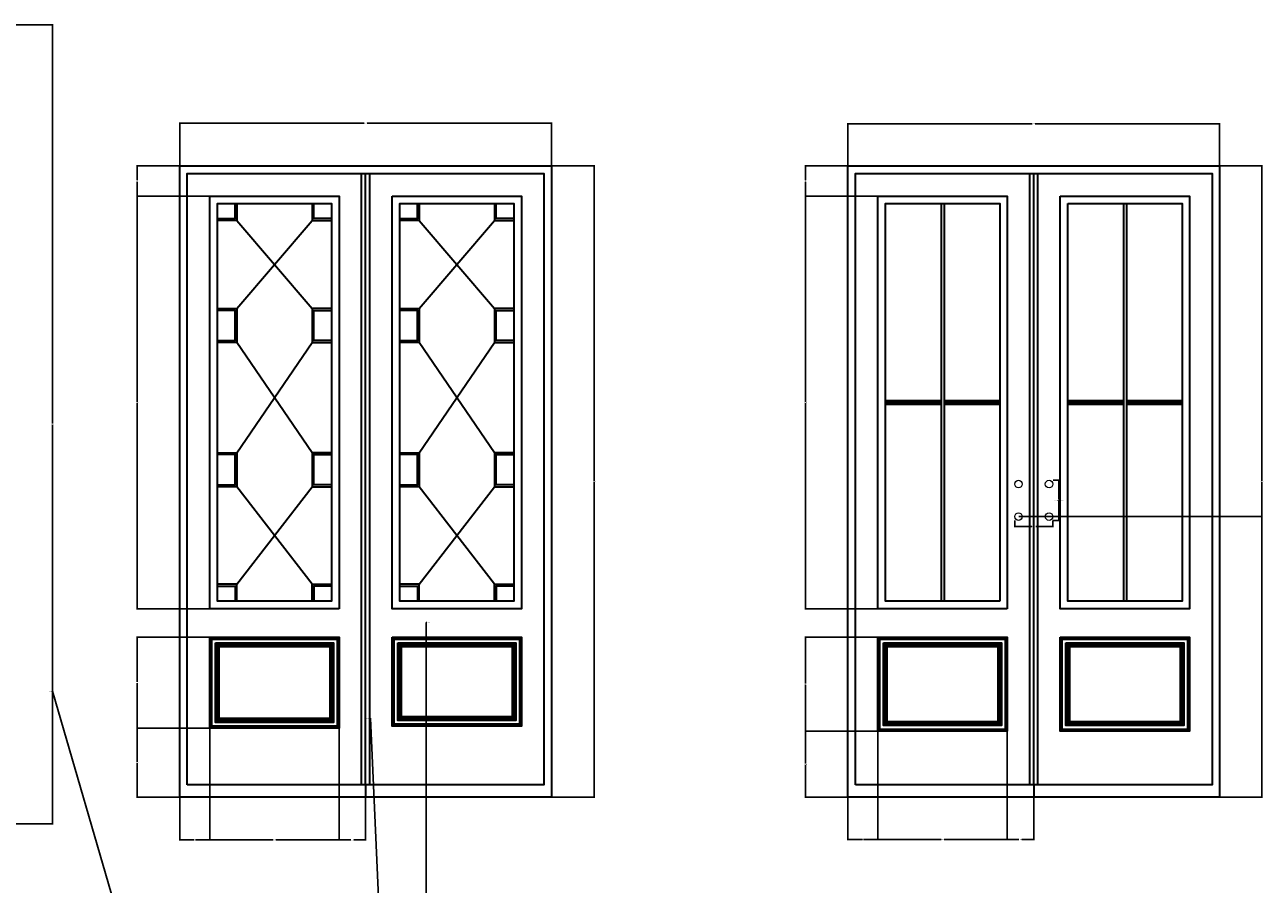
# Model space of a CAD drawing. Units: inches. Extents: x 1318 to 1980, y 617 to 1423.
# Tile 6 of 7: x 1650 to 1980, y 942 to 1170. Entities that reach past the tile are written whole.
import ezdxf

# ---------------------------------------------------------------- set-up
doc = ezdxf.new("R2010")
doc.units = ezdxf.units.IN
doc.header["$MEASUREMENT"] = 0
for name, color, linetype, lineweight in [('A-ANNO-DIMS', 2, 'Continuous', 18), ('A-DOOR', 4, 'Continuous', 35), ('A-DOOR-HDWR', 3, 'Continuous', 18)]:
    doc.layers.add(name, color=color, linetype=linetype, lineweight=lineweight)
doc.styles.get("Standard").update_dxf_attribs({"font": 'arial.ttf'})
doc.dimstyles.get("Standard").update_dxf_attribs({"dimtxt": 0.18, "dimasz": 0.18, "dimexe": 0.18, "dimexo": 0.0625, "dimgap": 0.09, "dimtad": 0, "dimtih": 1, "dimtoh": 1, "dimdec": 0, "dimzin": 0, "dimdsep": 46, "dimlunit": 3, "dimtxsty": 'Standard', "dimcen": 0.09, "dimadec": 0, "dimazin": 0, "dimtfac": 1, "dimtdec": 0, "dimtofl": 0, "dimtmove": 0, "dimatfit": 3, "dimfxl": 1, "dimtolj": 1, "dimtzin": 0, "dimarcsym": 0})

# ---------------------------------------------------------------- blocks, each defined once
blk = doc.blocks.new('DOOR-KNOB-SET')
for centre in [(1.01, 9.67), (9.16, 9.67), (1.01, 1.01), (9.16, 1.01)]:
    blk.add_circle(centre, 1.01)
blk = doc.blocks.new('*D2')
at = {"layer": 'A-ANNO-DIMS', "color": 0, "lineweight": -2, "transparency": 16777216}
for p, q in [((1923.71, 1049.16), (1925.43, 1049.16)), ((1925.25, 1048.98), (1925.25, 1044.01)), ((1925.25, 1038.66), (1925.25, 1043.64)), ((1923.71, 1038.48), (1925.43, 1038.48))]:
    blk.add_line(p, q, dxfattribs=at)
at = {"layer": 'A-ANNO-DIMS', "color": 0, "transparency": 16777216}
for points in [[(1925.22, 1048.98), (1925.28, 1048.98), (1925.25, 1049.16)], [(1925.22, 1038.66), (1925.28, 1038.66), (1925.25, 1038.48)]]:
    blk.add_solid(points, dxfattribs=at)
at = {"layer": 'Defpoints', "color": 0, "transparency": 16777216}
for p in [(1923.65, 1049.16), (1925.25, 1049.16), (1923.65, 1038.48)]:
    blk.add_point(p, dxfattribs=at)
at = {"layer": 'A-ANNO-DIMS', "color": 0, "transparency": 16777216, "insert": (1925.25, 1043.82), "char_height": 0.18, "attachment_point": 5}
blk.add_mtext('\\A1;DOOR KNOB SET 11 TYP.', dxfattribs=at)
blk = doc.blocks.new('*D3')
at = {"layer": 'A-ANNO-DIMS', "color": 0, "lineweight": -2, "transparency": 16777216}
for p, q in [((1913.49, 1038.42), (1913.49, 1036.7)), ((1913.67, 1036.88), (1918.05, 1036.88)), ((1923.47, 1036.88), (1919.09, 1036.88)), ((1923.65, 1038.42), (1923.65, 1036.7))]:
    blk.add_line(p, q, dxfattribs=at)
at = {"layer": 'A-ANNO-DIMS', "color": 0, "transparency": 16777216}
for points in [[(1913.67, 1036.91), (1913.67, 1036.85), (1913.49, 1036.88)], [(1923.47, 1036.91), (1923.47, 1036.85), (1923.65, 1036.88)]]:
    blk.add_solid(points, dxfattribs=at)
at = {"layer": 'Defpoints', "color": 0, "transparency": 16777216}
for p in [(1913.49, 1038.48), (1923.65, 1038.48), (1923.65, 1036.88)]:
    blk.add_point(p, dxfattribs=at)
at = {"layer": 'A-ANNO-DIMS', "color": 0, "transparency": 16777216, "insert": (1918.57, 1036.88), "char_height": 0.18, "attachment_point": 5}
blk.add_mtext('\\A1;10 TYP.', dxfattribs=at)
blk = doc.blocks.new('*D49')
at = {"layer": 'A-ANNO-DIMS', "color": 0, "lineweight": -2, "transparency": 16777216}
for p, q in [((1643.69, 1170.41), (1657.46, 1170.41)), ((1657.28, 1170.23), (1657.28, 1064.23)), ((1657.28, 957.88), (1657.28, 1063.87)), ((1643.69, 957.7), (1657.46, 957.7))]:
    blk.add_line(p, q, dxfattribs=at)
at = {"layer": 'A-ANNO-DIMS', "color": 0, "transparency": 16777216}
for points in [[(1657.25, 1170.23), (1657.31, 1170.23), (1657.28, 1170.41)], [(1657.25, 957.88), (1657.31, 957.88), (1657.28, 957.7)]]:
    blk.add_solid(points, dxfattribs=at)
at = {"layer": 'Defpoints', "color": 0, "transparency": 16777216}
for p in [(1643.63, 1170.41), (1657.28, 1170.41), (1643.63, 957.7)]:
    blk.add_point(p, dxfattribs=at)
at = {"layer": 'A-ANNO-DIMS', "color": 0, "transparency": 16777216, "insert": (1657.28, 1064.05), "char_height": 0.18, "attachment_point": 5}
blk.add_mtext('\\A1;212.7', dxfattribs=at)
blk = doc.blocks.new('*D57')
at = {"layer": 'A-ANNO-DIMS', "color": 0, "lineweight": -2, "transparency": 16777216}
for p, q in [((1691.16, 1132.88), (1691.16, 1144.4)), ((1691.34, 1144.22), (1740.25, 1144.22)), ((1789.95, 1144.22), (1741.04, 1144.22)), ((1790.13, 1132.88), (1790.13, 1144.4))]:
    blk.add_line(p, q, dxfattribs=at)
at = {"layer": 'A-ANNO-DIMS', "color": 0, "transparency": 16777216}
for points in [[(1691.34, 1144.25), (1691.34, 1144.19), (1691.16, 1144.22)], [(1789.95, 1144.25), (1789.95, 1144.19), (1790.13, 1144.22)]]:
    blk.add_solid(points, dxfattribs=at)
at = {"layer": 'Defpoints', "color": 0, "transparency": 16777216}
for p in [(1790.13, 1144.22), (1691.16, 1132.82), (1790.13, 1132.82)]:
    blk.add_point(p, dxfattribs=at)
at = {"layer": 'A-ANNO-DIMS', "color": 0, "transparency": 16777216, "insert": (1740.64, 1144.22), "char_height": 0.18, "attachment_point": 5}
blk.add_mtext('\\A1;98.98', dxfattribs=at)
blk = doc.blocks.new('*D58')
at = {"layer": 'A-ANNO-DIMS', "color": 0, "lineweight": -2, "transparency": 16777216}
for p, q in [((1790.2, 1132.82), (1801.71, 1132.82)), ((1801.53, 1132.64), (1801.53, 1048.99)), ((1801.53, 964.98), (1801.53, 1048.63)), ((1790.2, 964.8), (1801.71, 964.8))]:
    blk.add_line(p, q, dxfattribs=at)
at = {"layer": 'A-ANNO-DIMS', "color": 0, "transparency": 16777216}
for points in [[(1801.5, 1132.64), (1801.56, 1132.64), (1801.53, 1132.82)], [(1801.5, 964.98), (1801.56, 964.98), (1801.53, 964.8)]]:
    blk.add_solid(points, dxfattribs=at)
at = {"layer": 'Defpoints', "color": 0, "transparency": 16777216}
for p in [(1790.13, 1132.82), (1801.53, 1132.82), (1790.13, 964.8)]:
    blk.add_point(p, dxfattribs=at)
at = {"layer": 'A-ANNO-DIMS', "color": 0, "transparency": 16777216, "insert": (1801.53, 1048.81), "char_height": 0.18, "attachment_point": 5}
blk.add_mtext('\\A1;168.02', dxfattribs=at)
blk = doc.blocks.new('*D59')
at = {"layer": 'A-ANNO-DIMS', "color": 0, "lineweight": -2, "transparency": 16777216}
for p, q in [((1699.16, 983.13), (1699.16, 953.22)), ((1691.16, 964.73), (1691.16, 953.22)), ((1691.34, 953.4), (1695.01, 953.4)), ((1698.98, 953.4), (1695.3, 953.4))]:
    blk.add_line(p, q, dxfattribs=at)
at = {"layer": 'A-ANNO-DIMS', "color": 0, "transparency": 16777216}
for points in [[(1691.34, 953.43), (1691.34, 953.37), (1691.16, 953.4)], [(1698.98, 953.43), (1698.98, 953.37), (1699.16, 953.4)]]:
    blk.add_solid(points, dxfattribs=at)
at = {"layer": 'Defpoints', "color": 0, "transparency": 16777216}
for p in [(1699.16, 983.19), (1691.16, 964.8), (1699.16, 953.4)]:
    blk.add_point(p, dxfattribs=at)
at = {"layer": 'A-ANNO-DIMS', "color": 0, "transparency": 16777216, "insert": (1695.16, 953.4), "char_height": 0.18, "attachment_point": 5}
blk.add_mtext('\\A1;8', dxfattribs=at)
blk = doc.blocks.new('*D60')
at = {"layer": 'A-ANNO-DIMS', "color": 0, "lineweight": -2, "transparency": 16777216}
for p, q in [((1699.16, 983.13), (1699.16, 953.22)), ((1733.58, 983.13), (1733.58, 953.22)), ((1699.34, 953.4), (1715.97, 953.4)), ((1733.4, 953.4), (1716.76, 953.4))]:
    blk.add_line(p, q, dxfattribs=at)
at = {"layer": 'A-ANNO-DIMS', "color": 0, "transparency": 16777216}
for points in [[(1699.34, 953.43), (1699.34, 953.37), (1699.16, 953.4)], [(1733.4, 953.43), (1733.4, 953.37), (1733.58, 953.4)]]:
    blk.add_solid(points, dxfattribs=at)
at = {"layer": 'Defpoints', "color": 0, "transparency": 16777216}
for p in [(1699.16, 983.19), (1733.58, 983.19), (1733.58, 953.4)]:
    blk.add_point(p, dxfattribs=at)
at = {"layer": 'A-ANNO-DIMS', "color": 0, "transparency": 16777216, "insert": (1716.37, 953.4), "char_height": 0.18, "attachment_point": 5}
blk.add_mtext('\\A1;34.42', dxfattribs=at)
blk = doc.blocks.new('*D61')
at = {"layer": 'A-ANNO-DIMS', "color": 0, "lineweight": -2, "transparency": 16777216}
for p, q in [((1733.58, 983.13), (1733.58, 953.22)), ((1740.64, 964.73), (1740.64, 953.22)), ((1733.76, 953.4), (1736.72, 953.4)), ((1740.46, 953.4), (1737.5, 953.4))]:
    blk.add_line(p, q, dxfattribs=at)
at = {"layer": 'A-ANNO-DIMS', "color": 0, "transparency": 16777216}
for points in [[(1733.76, 953.43), (1733.76, 953.37), (1733.58, 953.4)], [(1740.46, 953.43), (1740.46, 953.37), (1740.64, 953.4)]]:
    blk.add_solid(points, dxfattribs=at)
at = {"layer": 'Defpoints', "color": 0, "transparency": 16777216}
for p in [(1733.58, 983.19), (1740.64, 964.8), (1740.64, 953.4)]:
    blk.add_point(p, dxfattribs=at)
at = {"layer": 'A-ANNO-DIMS', "color": 0, "transparency": 16777216, "insert": (1737.11, 953.4), "char_height": 0.18, "attachment_point": 5}
blk.add_mtext('\\A1;7.068', dxfattribs=at)
blk = doc.blocks.new('*D62')
at = {"layer": 'A-ANNO-DIMS', "color": 0, "lineweight": -2, "transparency": 16777216}
for p, q in [((1699.09, 983.19), (1679.58, 983.19)), ((1679.76, 983.01), (1679.76, 974.18)), ((1679.76, 964.98), (1679.76, 973.81)), ((1691.09, 964.8), (1679.58, 964.8))]:
    blk.add_line(p, q, dxfattribs=at)
at = {"layer": 'A-ANNO-DIMS', "color": 0, "transparency": 16777216}
for points in [[(1679.73, 983.01), (1679.79, 983.01), (1679.76, 983.19)], [(1679.73, 964.98), (1679.79, 964.98), (1679.76, 964.8)]]:
    blk.add_solid(points, dxfattribs=at)
at = {"layer": 'Defpoints', "color": 0, "transparency": 16777216}
for p in [(1679.76, 983.19), (1699.16, 983.19), (1691.16, 964.8)]:
    blk.add_point(p, dxfattribs=at)
at = {"layer": 'A-ANNO-DIMS', "color": 0, "transparency": 16777216, "insert": (1679.76, 973.99), "char_height": 0.18, "attachment_point": 5}
blk.add_mtext('\\A1;18.395', dxfattribs=at)
blk = doc.blocks.new('*D63')
at = {"layer": 'A-ANNO-DIMS', "color": 0, "lineweight": -2, "transparency": 16777216}
for p, q in [((1699.09, 1007.37), (1679.58, 1007.37)), ((1679.76, 1007.19), (1679.76, 995.46)), ((1679.76, 983.37), (1679.76, 995.1)), ((1699.09, 983.19), (1679.58, 983.19))]:
    blk.add_line(p, q, dxfattribs=at)
at = {"layer": 'A-ANNO-DIMS', "color": 0, "transparency": 16777216}
for points in [[(1679.73, 1007.19), (1679.79, 1007.19), (1679.76, 1007.37)], [(1679.73, 983.37), (1679.79, 983.37), (1679.76, 983.19)]]:
    blk.add_solid(points, dxfattribs=at)
at = {"layer": 'Defpoints', "color": 0, "transparency": 16777216}
for p in [(1679.76, 1007.37), (1699.16, 1007.37), (1699.16, 983.19)]:
    blk.add_point(p, dxfattribs=at)
at = {"layer": 'A-ANNO-DIMS', "color": 0, "transparency": 16777216, "insert": (1679.76, 995.28), "char_height": 0.18, "attachment_point": 5}
blk.add_mtext('\\A1;24.18', dxfattribs=at)
blk = doc.blocks.new('*D64')
at = {"layer": 'A-ANNO-DIMS', "color": 0, "lineweight": -2, "transparency": 16777216}
for p, q in [((1699.09, 1124.82), (1679.58, 1124.82)), ((1679.76, 1124.64), (1679.76, 1070.07)), ((1679.76, 1015.13), (1679.76, 1069.7)), ((1699.09, 1014.95), (1679.58, 1014.95))]:
    blk.add_line(p, q, dxfattribs=at)
at = {"layer": 'A-ANNO-DIMS', "color": 0, "transparency": 16777216}
for points in [[(1679.73, 1124.64), (1679.79, 1124.64), (1679.76, 1124.82)], [(1679.73, 1015.13), (1679.79, 1015.13), (1679.76, 1014.95)]]:
    blk.add_solid(points, dxfattribs=at)
at = {"layer": 'Defpoints', "color": 0, "transparency": 16777216}
for p in [(1679.76, 1124.82), (1699.16, 1124.82), (1699.16, 1014.95)]:
    blk.add_point(p, dxfattribs=at)
at = {"layer": 'A-ANNO-DIMS', "color": 0, "transparency": 16777216, "insert": (1679.76, 1069.89), "char_height": 0.18, "attachment_point": 5}
blk.add_mtext('\\A1;109.87', dxfattribs=at)
blk = doc.blocks.new('*D65')
at = {"layer": 'A-ANNO-DIMS', "color": 0, "lineweight": -2, "transparency": 16777216}
for p, q in [((1691.09, 1132.82), (1679.58, 1132.82)), ((1679.76, 1132.64), (1679.76, 1129)), ((1679.76, 1125), (1679.76, 1128.64)), ((1699.09, 1124.82), (1679.58, 1124.82))]:
    blk.add_line(p, q, dxfattribs=at)
at = {"layer": 'A-ANNO-DIMS', "color": 0, "transparency": 16777216}
for points in [[(1679.73, 1132.64), (1679.79, 1132.64), (1679.76, 1132.82)], [(1679.73, 1125), (1679.79, 1125), (1679.76, 1124.82)]]:
    blk.add_solid(points, dxfattribs=at)
at = {"layer": 'Defpoints', "color": 0, "transparency": 16777216}
for p in [(1679.76, 1132.82), (1691.16, 1132.82), (1699.16, 1124.82)]:
    blk.add_point(p, dxfattribs=at)
at = {"layer": 'A-ANNO-DIMS', "color": 0, "transparency": 16777216, "insert": (1679.76, 1128.82), "char_height": 0.18, "attachment_point": 5}
blk.add_mtext('\\A1;8', dxfattribs=at)
blk = doc.blocks.new('*D66')
at = {"layer": 'A-ANNO-DIMS', "color": 0, "lineweight": -2, "transparency": 16777216}
for p, q in [((1914.558836, 1039.490656), (1979.476261, 1039.490656)), ((1979.296261, 1039.310656), (1979.296261, 1002.323284)), ((1979.296261, 964.975912), (1979.296261, 1001.963284)), ((1918.619524, 964.795912), (1979.476261, 964.795912))]:
    blk.add_line(p, q, dxfattribs=at)
at = {"layer": 'A-ANNO-DIMS', "color": 0, "transparency": 16777216}
for points in [[(1979.266261, 1039.310656), (1979.326261, 1039.310656), (1979.296261, 1039.490656)], [(1979.266261, 964.975912), (1979.326261, 964.975912), (1979.296261, 964.795912)]]:
    blk.add_solid(points, dxfattribs=at)
at = {"layer": 'Defpoints', "color": 0, "transparency": 16777216}
for p in [(1914.496336, 1039.490656), (1979.296261, 1039.490656), (1918.557024, 964.795912)]:
    blk.add_point(p, dxfattribs=at)
at = {"layer": 'A-ANNO-DIMS', "color": 0, "transparency": 16777216, "insert": (1979.296261, 1002.143284), "char_height": 0.18, "attachment_point": 5}
blk.add_mtext('\\A1;74.7', dxfattribs=at)
blk = doc.blocks.new('*D67')
at = {"layer": 'A-ANNO-DIMS', "color": 0, "lineweight": -2, "transparency": 16777216}
for p, q in [((1869.07, 1132.88), (1869.07, 1144.25)), ((1869.25, 1144.07), (1918.16, 1144.07)), ((1967.87, 1144.07), (1918.95, 1144.07)), ((1968.05, 1132.88), (1968.05, 1144.25))]:
    blk.add_line(p, q, dxfattribs=at)
at = {"layer": 'A-ANNO-DIMS', "color": 0, "transparency": 16777216}
for points in [[(1869.25, 1144.1), (1869.25, 1144.04), (1869.07, 1144.07)], [(1967.87, 1144.1), (1967.87, 1144.04), (1968.05, 1144.07)]]:
    blk.add_solid(points, dxfattribs=at)
at = {"layer": 'Defpoints', "color": 0, "transparency": 16777216}
for p in [(1968.05, 1144.07), (1869.07, 1132.82), (1968.05, 1132.82)]:
    blk.add_point(p, dxfattribs=at)
at = {"layer": 'A-ANNO-DIMS', "color": 0, "transparency": 16777216, "insert": (1918.56, 1144.07), "char_height": 0.18, "attachment_point": 5}
blk.add_mtext('\\A1;98.98', dxfattribs=at)
blk = doc.blocks.new('*D68')
at = {"layer": 'A-ANNO-DIMS', "color": 0, "lineweight": -2, "transparency": 16777216}
for p, q in [((1968.11, 1132.82), (1979.48, 1132.82)), ((1979.3, 1132.64), (1979.3, 1048.99)), ((1979.3, 964.98), (1979.3, 1048.63)), ((1968.11, 964.8), (1979.48, 964.8))]:
    blk.add_line(p, q, dxfattribs=at)
at = {"layer": 'A-ANNO-DIMS', "color": 0, "transparency": 16777216}
for points in [[(1979.27, 1132.64), (1979.33, 1132.64), (1979.3, 1132.82)], [(1979.27, 964.98), (1979.33, 964.98), (1979.3, 964.8)]]:
    blk.add_solid(points, dxfattribs=at)
at = {"layer": 'Defpoints', "color": 0, "transparency": 16777216}
for p in [(1968.05, 1132.82), (1979.3, 1132.82), (1968.05, 964.8)]:
    blk.add_point(p, dxfattribs=at)
at = {"layer": 'A-ANNO-DIMS', "color": 0, "transparency": 16777216, "insert": (1979.3, 1048.81), "char_height": 0.18, "attachment_point": 5}
blk.add_mtext('\\A1;168.02', dxfattribs=at)
blk = doc.blocks.new('*D69')
at = {"layer": 'A-ANNO-DIMS', "color": 0, "lineweight": -2, "transparency": 16777216}
for p, q in [((1877.07, 982.26), (1877.07, 953.37)), ((1869.07, 964.73), (1869.07, 953.37)), ((1869.25, 953.55), (1872.92, 953.55)), ((1876.89, 953.55), (1873.22, 953.55))]:
    blk.add_line(p, q, dxfattribs=at)
at = {"layer": 'A-ANNO-DIMS', "color": 0, "transparency": 16777216}
for points in [[(1869.25, 953.58), (1869.25, 953.52), (1869.07, 953.55)], [(1876.89, 953.58), (1876.89, 953.52), (1877.07, 953.55)]]:
    blk.add_solid(points, dxfattribs=at)
at = {"layer": 'Defpoints', "color": 0, "transparency": 16777216}
for p in [(1877.07, 982.33), (1869.07, 964.8), (1877.07, 953.55)]:
    blk.add_point(p, dxfattribs=at)
at = {"layer": 'A-ANNO-DIMS', "color": 0, "transparency": 16777216, "insert": (1873.07, 953.55), "char_height": 0.18, "attachment_point": 5}
blk.add_mtext('\\A1;8', dxfattribs=at)
blk = doc.blocks.new('*D70')
at = {"layer": 'A-ANNO-DIMS', "color": 0, "lineweight": -2, "transparency": 16777216}
for p, q in [((1877.07, 982.26), (1877.07, 953.37)), ((1911.49, 982.26), (1911.49, 953.37)), ((1877.25, 953.55), (1893.89, 953.55)), ((1911.31, 953.55), (1894.67, 953.55))]:
    blk.add_line(p, q, dxfattribs=at)
at = {"layer": 'A-ANNO-DIMS', "color": 0, "transparency": 16777216}
for points in [[(1877.25, 953.58), (1877.25, 953.52), (1877.07, 953.55)], [(1911.31, 953.58), (1911.31, 953.52), (1911.49, 953.55)]]:
    blk.add_solid(points, dxfattribs=at)
at = {"layer": 'Defpoints', "color": 0, "transparency": 16777216}
for p in [(1877.07, 982.33), (1911.49, 982.33), (1911.49, 953.55)]:
    blk.add_point(p, dxfattribs=at)
at = {"layer": 'A-ANNO-DIMS', "color": 0, "transparency": 16777216, "insert": (1894.28, 953.55), "char_height": 0.18, "attachment_point": 5}
blk.add_mtext('\\A1;34.42', dxfattribs=at)
blk = doc.blocks.new('*D71')
at = {"layer": 'A-ANNO-DIMS', "color": 0, "lineweight": -2, "transparency": 16777216}
for p, q in [((1911.49, 982.26), (1911.49, 953.37)), ((1918.56, 964.73), (1918.56, 953.37)), ((1911.67, 953.55), (1914.63, 953.55)), ((1918.38, 953.55), (1915.42, 953.55))]:
    blk.add_line(p, q, dxfattribs=at)
at = {"layer": 'A-ANNO-DIMS', "color": 0, "transparency": 16777216}
for points in [[(1911.67, 953.58), (1911.67, 953.52), (1911.49, 953.55)], [(1918.38, 953.58), (1918.38, 953.52), (1918.56, 953.55)]]:
    blk.add_solid(points, dxfattribs=at)
at = {"layer": 'Defpoints', "color": 0, "transparency": 16777216}
for p in [(1911.49, 982.33), (1918.56, 964.8), (1918.56, 953.55)]:
    blk.add_point(p, dxfattribs=at)
at = {"layer": 'A-ANNO-DIMS', "color": 0, "transparency": 16777216, "insert": (1915.02, 953.55), "char_height": 0.18, "attachment_point": 5}
blk.add_mtext('\\A1;7.068', dxfattribs=at)
blk = doc.blocks.new('*D72')
at = {"layer": 'A-ANNO-DIMS', "color": 0, "lineweight": -2, "transparency": 16777216}
for p, q in [((1877.01, 982.33), (1857.64, 982.33)), ((1857.82, 982.15), (1857.82, 973.74)), ((1857.82, 964.98), (1857.82, 973.38)), ((1869.01, 964.8), (1857.64, 964.8))]:
    blk.add_line(p, q, dxfattribs=at)
at = {"layer": 'A-ANNO-DIMS', "color": 0, "transparency": 16777216}
for points in [[(1857.79, 982.15), (1857.85, 982.15), (1857.82, 982.33)], [(1857.79, 964.98), (1857.85, 964.98), (1857.82, 964.8)]]:
    blk.add_solid(points, dxfattribs=at)
at = {"layer": 'Defpoints', "color": 0, "transparency": 16777216}
for p in [(1857.82, 982.33), (1877.07, 982.33), (1869.07, 964.8)]:
    blk.add_point(p, dxfattribs=at)
at = {"layer": 'A-ANNO-DIMS', "color": 0, "transparency": 16777216, "insert": (1857.82, 973.56), "char_height": 0.18, "attachment_point": 5}
blk.add_mtext('\\A1;17.53', dxfattribs=at)
blk = doc.blocks.new('*D73')
at = {"layer": 'A-ANNO-DIMS', "color": 0, "lineweight": -2, "transparency": 16777216}
for p, q in [((1877.01, 1007.37), (1857.64, 1007.37)), ((1857.82, 1007.19), (1857.82, 995.03)), ((1857.82, 982.51), (1857.82, 994.67)), ((1877.01, 982.33), (1857.64, 982.33))]:
    blk.add_line(p, q, dxfattribs=at)
at = {"layer": 'A-ANNO-DIMS', "color": 0, "transparency": 16777216}
for points in [[(1857.79, 1007.19), (1857.85, 1007.19), (1857.82, 1007.37)], [(1857.79, 982.51), (1857.85, 982.51), (1857.82, 982.33)]]:
    blk.add_solid(points, dxfattribs=at)
at = {"layer": 'Defpoints', "color": 0, "transparency": 16777216}
for p in [(1857.82, 1007.37), (1877.07, 1007.37), (1877.07, 982.33)]:
    blk.add_point(p, dxfattribs=at)
at = {"layer": 'A-ANNO-DIMS', "color": 0, "transparency": 16777216, "insert": (1857.82, 994.85), "char_height": 0.18, "attachment_point": 5}
blk.add_mtext('\\A1;25.044', dxfattribs=at)
blk = doc.blocks.new('*D74')
at = {"layer": 'A-ANNO-DIMS', "color": 0, "lineweight": -2, "transparency": 16777216}
for p, q in [((1877.01, 1124.82), (1857.64, 1124.82)), ((1857.82, 1124.64), (1857.82, 1070.07)), ((1857.82, 1015.13), (1857.82, 1069.7)), ((1877.01, 1014.95), (1857.64, 1014.95))]:
    blk.add_line(p, q, dxfattribs=at)
at = {"layer": 'A-ANNO-DIMS', "color": 0, "transparency": 16777216}
for points in [[(1857.79, 1124.64), (1857.85, 1124.64), (1857.82, 1124.82)], [(1857.79, 1015.13), (1857.85, 1015.13), (1857.82, 1014.95)]]:
    blk.add_solid(points, dxfattribs=at)
at = {"layer": 'Defpoints', "color": 0, "transparency": 16777216}
for p in [(1857.82, 1124.82), (1877.07, 1124.82), (1877.07, 1014.95)]:
    blk.add_point(p, dxfattribs=at)
at = {"layer": 'A-ANNO-DIMS', "color": 0, "transparency": 16777216, "insert": (1857.82, 1069.89), "char_height": 0.18, "attachment_point": 5}
blk.add_mtext('\\A1;109.87', dxfattribs=at)
blk = doc.blocks.new('*D75')
at = {"layer": 'A-ANNO-DIMS', "color": 0, "lineweight": -2, "transparency": 16777216}
for p, q in [((1869.01, 1132.82), (1857.64, 1132.82)), ((1857.82, 1132.64), (1857.82, 1129)), ((1857.82, 1125), (1857.82, 1128.64)), ((1877.01, 1124.82), (1857.64, 1124.82))]:
    blk.add_line(p, q, dxfattribs=at)
at = {"layer": 'A-ANNO-DIMS', "color": 0, "transparency": 16777216}
for points in [[(1857.79, 1132.64), (1857.85, 1132.64), (1857.82, 1132.82)], [(1857.79, 1125), (1857.85, 1125), (1857.82, 1124.82)]]:
    blk.add_solid(points, dxfattribs=at)
at = {"layer": 'Defpoints', "color": 0, "transparency": 16777216}
for p in [(1857.82, 1132.82), (1869.07, 1132.82), (1877.07, 1124.82)]:
    blk.add_point(p, dxfattribs=at)
at = {"layer": 'A-ANNO-DIMS', "color": 0, "transparency": 16777216, "insert": (1857.82, 1128.82), "char_height": 0.18, "attachment_point": 5}
blk.add_mtext('\\A1;8', dxfattribs=at)
blk = doc.blocks.new('*D114')
at = {"layer": 'A-ANNO-DIMS', "color": 0, "lineweight": -2, "transparency": 16777216}
for p, q in [((1922.55, 1039.49), (1922.73, 1039.49)), ((1922.64, 1039.4), (1922.64, 1039.58)), ((1924.26, 1039.51), (1923.83, 1039.5))]:
    blk.add_line(p, q, dxfattribs=at)
at = {"layer": 'A-ANNO-DIMS', "color": 0, "transparency": 16777216}
blk.add_solid([(1923.83, 1039.53), (1923.83, 1039.47), (1923.65, 1039.5)], dxfattribs=at)
at = {"layer": 'Defpoints', "color": 0, "transparency": 16777216}
for p in [(1921.63, 1039.48), (1923.65, 1039.5)]:
    blk.add_point(p, dxfattribs=at)
at = {"layer": 'A-ANNO-DIMS', "color": 0, "transparency": 16777216, "insert": (1924.94, 1039.51), "char_height": 0.18, "attachment_point": 5}
blk.add_mtext('\\A1;4X ∅2.017', dxfattribs=at)
blk = doc.blocks.new('*D118')
at = {"layer": 'A-ANNO-DIMS', "color": 0, "lineweight": -2, "transparency": 16777216}
for p, q in [((1756.97, 1011.3), (1756.79, 1011.3)), ((1756.79, 1011.3), (1756.79, 875.96)), ((1756.7, 649.9), (1756.88, 649.9)), ((1756.79, 649.81), (1756.79, 649.99))]:
    blk.add_line(p, q, dxfattribs=at)
at = {"layer": 'A-ANNO-DIMS', "color": 0, "transparency": 16777216}
blk.add_solid([(1756.76, 875.96), (1756.82, 875.96), (1756.79, 875.78)], dxfattribs=at)
at = {"layer": 'Defpoints', "color": 0, "transparency": 16777216}
for p in [(1756.79, 875.78), (1756.79, 649.9)]:
    blk.add_point(p, dxfattribs=at)
at = {"layer": 'A-ANNO-DIMS', "color": 0, "transparency": 16777216, "insert": (1757.45, 1011.3), "char_height": 0.18, "attachment_point": 5}
blk.add_mtext('\\A1;R225.9', dxfattribs=at)
blk = doc.blocks.new('*D119')
at = {"layer": 'A-ANNO-DIMS', "color": 0, "lineweight": -2, "transparency": 16777216}
for p, q in [((1657.1, 992.97), (1657.28, 992.97)), ((1657.28, 992.97), (1694.55, 864.49)), ((1756.7, 649.9), (1756.88, 649.9)), ((1756.79, 649.81), (1756.79, 649.99))]:
    blk.add_line(p, q, dxfattribs=at)
at = {"layer": 'A-ANNO-DIMS', "color": 0, "transparency": 16777216}
blk.add_solid([(1694.57, 864.5), (1694.52, 864.48), (1694.6, 864.32)], dxfattribs=at)
at = {"layer": 'Defpoints', "color": 0, "transparency": 16777216}
for p in [(1694.6, 864.32), (1756.79, 649.9)]:
    blk.add_point(p, dxfattribs=at)
at = {"layer": 'A-ANNO-DIMS', "color": 0, "transparency": 16777216, "insert": (1656.55, 992.97), "char_height": 0.18, "attachment_point": 5}
blk.add_mtext('\\A1;R223.26', dxfattribs=at)
blk = doc.blocks.new('*D120')
at = {"layer": 'A-ANNO-DIMS', "color": 0, "lineweight": -2, "transparency": 16777216}
for p, q in [((1741.75, 985.8), (1741.93, 985.8)), ((1741.93, 985.8), (1747.49, 860.02)), ((1756.7, 649.9), (1756.88, 649.9)), ((1756.79, 649.81), (1756.79, 649.99))]:
    blk.add_line(p, q, dxfattribs=at)
at = {"layer": 'A-ANNO-DIMS', "color": 0, "transparency": 16777216}
blk.add_solid([(1747.52, 860.02), (1747.46, 860.02), (1747.5, 859.84)], dxfattribs=at)
at = {"layer": 'Defpoints', "color": 0, "transparency": 16777216}
for p in [(1747.5, 859.84), (1756.79, 649.9)]:
    blk.add_point(p, dxfattribs=at)
at = {"layer": 'A-ANNO-DIMS', "color": 0, "transparency": 16777216, "insert": (1741, 985.8), "char_height": 0.18, "attachment_point": 5}
blk.add_mtext('\\A1;4X R210.15', dxfattribs=at)

msp = doc.modelspace()

# ---------------------------------------------------------------- linework, layer by layer
at = {"layer": 'A-DOOR'}
for p, q in [((1739.5765, 968.0892), (1739.5765, 1130.8191)), ((1740.6445, 968.0892), (1740.6445, 1130.8191)), ((1741.7125, 968.0892), (1741.7125, 1130.8191)), ((1917.4891, 968.0892), (1917.4891, 1130.8191)), ((1918.557, 968.0892), (1918.557, 1130.8191)), ((1919.625, 968.0892), (1919.625, 1130.8191)), ((1893.8845, 1122.8191), (1893.8845, 1016.9539)), ((1894.7081, 1122.8191), (1894.7081, 1016.9539)), ((1942.4417, 1122.8191), (1942.4417, 1016.9539)), ((1943.2653, 1122.8191), (1943.2653, 1016.9539)), ((1706.3574, 1094.8725), (1726.3743, 1118.3047)), ((1706.3574, 1118.3047), (1726.3743, 1094.8725)), ((1754.9146, 1118.3047), (1774.9315, 1094.8725)), ((1754.9146, 1094.8725), (1774.9315, 1118.3047)), ((1706.3574, 1056.475), (1726.3743, 1085.8437)), ((1726.3743, 1056.475), (1706.3574, 1085.8437)), ((1754.9146, 1056.475), (1774.9315, 1085.8437)), ((1774.9315, 1056.475), (1754.9146, 1085.8437)), ((1879.0678, 1070.3865), (1893.8845, 1070.3865)), ((1879.0678, 1069.8865), (1893.8845, 1069.8865)), ((1879.0678, 1069.3865), (1893.8845, 1069.3865)), ((1894.7081, 1070.3865), (1909.4891, 1070.3865)), ((1894.7081, 1069.8865), (1909.4891, 1069.8865)), ((1894.7081, 1069.3865), (1909.4891, 1069.3865)), ((1927.625, 1070.3865), (1942.4417, 1070.3865)), ((1927.625, 1069.8865), (1942.4417, 1069.8865)), ((1927.625, 1069.3865), (1942.4417, 1069.3865)), ((1943.2653, 1070.3865), (1958.0463, 1070.3865)), ((1943.2653, 1069.8865), (1958.0463, 1069.8865)), ((1943.2653, 1069.3865), (1958.0463, 1069.3865)), ((1706.3574, 1021.4683), (1726.3743, 1047.4462)), ((1726.3743, 1021.4683), (1706.3574, 1047.4462)), ((1754.9146, 1021.4683), (1774.9315, 1047.4462)), ((1774.9315, 1021.4683), (1754.9146, 1047.4462)), ((1699.1552, 1007.3699), (1699.6552, 1006.8699)), ((1733.0765, 1006.8699), (1733.5765, 1007.3699)), ((1747.7125, 1007.3699), (1748.2125, 1006.8699)), ((1781.6337, 1006.8699), (1782.1337, 1007.3699)), ((1877.0678, 1007.3699), (1877.5678, 1006.8699)), ((1910.9891, 1006.8699), (1911.4891, 1007.3699)), ((1925.625, 1007.3699), (1926.125, 1006.8699)), ((1959.5463, 1006.8699), (1960.0463, 1007.3699)), ((1700.6552, 1005.8699), (1701.6552, 1004.8699)), ((1731.0765, 1004.8699), (1732.0765, 1005.8699)), ((1749.2125, 1005.8699), (1750.2125, 1004.8699)), ((1779.6337, 1004.8699), (1780.6337, 1005.8699)), ((1878.5678, 1005.8699), (1879.5678, 1004.8699)), ((1908.9891, 1004.8699), (1909.9891, 1005.8699)), ((1927.125, 1005.8699), (1928.125, 1004.8699)), ((1957.5463, 1004.8699), (1958.5463, 1005.8699)), ((1749.2125, 985.1905), (1750.2125, 986.1905)), ((1780.6337, 985.1905), (1779.6337, 986.1905)), ((1699.1552, 983.1905), (1699.6552, 983.6905)), ((1700.6552, 984.6905), (1701.6552, 985.6905)), ((1732.0765, 984.6905), (1731.0765, 985.6905)), ((1733.5765, 983.1905), (1733.0765, 983.6905)), ((1747.7125, 983.6905), (1748.2125, 984.1905)), ((1782.1337, 983.6905), (1781.6337, 984.1905)), ((1877.0678, 982.3255), (1877.5678, 982.8255)), ((1878.5678, 983.8255), (1879.5678, 984.8255)), ((1909.9891, 983.8255), (1908.9891, 984.8255)), ((1911.4891, 982.3255), (1910.9891, 982.8255)), ((1925.625, 982.3255), (1926.125, 982.8255)), ((1927.125, 983.8255), (1928.125, 984.8255)), ((1958.5463, 983.8255), (1957.5463, 984.8255)), ((1960.0463, 982.3255), (1959.5463, 982.8255)), ((1740.6445, 968.0892), (1740.6445, 964.7959)), ((1918.557, 968.0892), (1918.557, 964.7959))]:
    msp.add_line(p, q, dxfattribs=at)
for points in [[(1691.1552, 1132.8191), (1790.1337, 1132.8191), (1790.1337, 964.7959), (1691.1552, 964.7959)], [(1869.0678, 1132.8191), (1968.0463, 1132.8191), (1968.0463, 964.7959), (1869.0678, 964.7959)], [(1693.1552, 968.0892), (1693.1552, 1130.8191), (1788.1337, 1130.8191), (1788.1337, 968.0892)], [(1871.0678, 968.0892), (1871.0678, 1130.8191), (1966.0463, 1130.8191), (1966.0463, 968.0892)], [(1733.5765, 1014.9539), (1699.1552, 1014.9539), (1699.1552, 1124.8191), (1733.5765, 1124.8191)], [(1747.7125, 1124.8191), (1782.1337, 1124.8191), (1782.1337, 1014.9539), (1747.7125, 1014.9539)], [(1911.4891, 1014.9539), (1877.0678, 1014.9539), (1877.0678, 1124.8191), (1911.4891, 1124.8191)], [(1925.625, 1124.8191), (1960.0463, 1124.8191), (1960.0463, 1014.9539), (1925.625, 1014.9539)], [(1909.4891, 1016.9539), (1879.0678, 1016.9539), (1879.0678, 1122.8191), (1909.4891, 1122.8191)], [(1927.625, 1122.8191), (1958.0463, 1122.8191), (1958.0463, 1016.9539), (1927.625, 1016.9539)], [(1699.1552, 1007.3699), (1733.5765, 1007.3699), (1733.5765, 983.1905), (1699.1552, 983.1905)], [(1699.6552, 1006.8699), (1733.0765, 1006.8699), (1733.0765, 983.6905), (1699.6552, 983.6905)], [(1747.7125, 1007.3699), (1782.1337, 1007.3699), (1782.1337, 983.6905), (1747.7125, 983.6905)], [(1748.2125, 1006.8699), (1781.6337, 1006.8699), (1781.6337, 984.1905), (1748.2125, 984.1905)], [(1877.0678, 1007.3699), (1911.4891, 1007.3699), (1911.4891, 982.3255), (1877.0678, 982.3255)], [(1877.5678, 1006.8699), (1910.9891, 1006.8699), (1910.9891, 982.8255), (1877.5678, 982.8255)], [(1925.625, 1007.3699), (1960.0463, 1007.3699), (1960.0463, 982.3255), (1925.625, 982.3255)], [(1926.125, 1006.8699), (1959.5463, 1006.8699), (1959.5463, 982.8255), (1926.125, 982.8255)], [(1700.6552, 1005.8699), (1732.0765, 1005.8699), (1732.0765, 984.6905), (1700.6552, 984.6905)], [(1701.1552, 1005.3699), (1731.5765, 1005.3699), (1731.5765, 985.1905), (1701.1552, 985.1905)], [(1701.6552, 1004.8699), (1731.0765, 1004.8699), (1731.0765, 985.6905), (1701.6552, 985.6905)], [(1749.2125, 1005.8699), (1780.6337, 1005.8699), (1780.6337, 985.1905), (1749.2125, 985.1905)], [(1749.7125, 1005.3699), (1780.1337, 1005.3699), (1780.1337, 985.6905), (1749.7125, 985.6905)], [(1750.2125, 1004.8699), (1779.6337, 1004.8699), (1779.6337, 986.1905), (1750.2125, 986.1905)], [(1878.5678, 1005.8699), (1909.9891, 1005.8699), (1909.9891, 983.8255), (1878.5678, 983.8255)], [(1879.0678, 1005.3699), (1909.4891, 1005.3699), (1909.4891, 984.3255), (1879.0678, 984.3255)], [(1879.5678, 1004.8699), (1908.9891, 1004.8699), (1908.9891, 984.8255), (1879.5678, 984.8255)], [(1927.125, 1005.8699), (1958.5463, 1005.8699), (1958.5463, 983.8255), (1927.125, 983.8255)], [(1927.625, 1005.3699), (1958.0463, 1005.3699), (1958.0463, 984.3255), (1927.625, 984.3255)], [(1928.125, 1004.8699), (1957.5463, 1004.8699), (1957.5463, 984.8255), (1928.125, 984.8255)]]:
    msp.add_lwpolyline(points, close=True, dxfattribs=at)
for points in [[(1731.5765, 1122.8191), (1731.5765, 1016.9539), (1701.1552, 1016.9539), (1701.1552, 1122.8191)], [(1701.1552, 1043.5636), (1701.1552, 1122.8191)], [(1701.1552, 1070.3865), (1701.1552, 1122.8191)], [(1701.1552, 1095.8725), (1701.1552, 1122.8191), (1731.5765, 1122.8191), (1731.5765, 1095.8725)], [(1706.3574, 1122.8191), (1706.3574, 1118.8047), (1706.3574, 1118.3047), (1705.8574, 1118.3047), (1701.1552, 1118.3047)], [(1701.1552, 1118.8047), (1705.8574, 1118.8047), (1705.8574, 1122.8191)], [(1726.3743, 1122.8191), (1726.3743, 1118.8047), (1726.3743, 1118.3047), (1726.8743, 1118.3047), (1731.5765, 1118.3047)], [(1731.5765, 1118.8047), (1726.8743, 1118.8047), (1726.8743, 1122.8191)], [(1731.5765, 1122.8191), (1731.5765, 1070.3865)], [(1731.5765, 1122.8191), (1731.5765, 1043.5636)], [(1749.7125, 1095.8725), (1749.7125, 1122.8191), (1780.1337, 1122.8191), (1780.1337, 1095.8725)], [(1780.1337, 1122.8191), (1780.1337, 1016.9539), (1749.7125, 1016.9539), (1749.7125, 1122.8191)], [(1754.9146, 1122.8191), (1754.9146, 1118.8047), (1754.9146, 1118.3047), (1754.4146, 1118.3047), (1749.7125, 1118.3047)], [(1749.7125, 1118.8047), (1754.4146, 1118.8047), (1754.4146, 1122.8191)], [(1774.9315, 1122.8191), (1774.9315, 1118.8047), (1774.9315, 1118.3047), (1775.4315, 1118.3047), (1780.1337, 1118.3047)], [(1780.1337, 1118.8047), (1775.4315, 1118.8047), (1775.4315, 1122.8191)], [(1701.1552, 1094.8725), (1705.8574, 1094.8725), (1706.3574, 1094.8725), (1706.3574, 1094.3725), (1706.3574, 1090.3581), (1706.3574, 1086.3437), (1706.3574, 1085.8437), (1705.8574, 1085.8437), (1701.1552, 1085.8437)], [(1701.1552, 1086.3437), (1705.8574, 1086.3437), (1705.8574, 1090.3581), (1705.8574, 1094.3725), (1701.1552, 1094.3725)], [(1731.5765, 1094.8725), (1726.8743, 1094.8725), (1726.3743, 1094.8725), (1726.3743, 1094.3725), (1726.3743, 1090.3581), (1726.3743, 1086.3437), (1726.3743, 1085.8437), (1726.8743, 1085.8437), (1731.5765, 1085.8437)], [(1731.5765, 1086.3437), (1726.8743, 1086.3437), (1726.8743, 1090.3581), (1726.8743, 1094.3725), (1731.5765, 1094.3725)], [(1749.7125, 1070.3865), (1749.7125, 1094.8725)], [(1749.7125, 1094.8725), (1754.4146, 1094.8725), (1754.9146, 1094.8725), (1754.9146, 1094.3725), (1754.9146, 1090.3581), (1754.9146, 1086.3437), (1754.9146, 1085.8437), (1754.4146, 1085.8437), (1749.7125, 1085.8437)], [(1749.7125, 1086.3437), (1754.4146, 1086.3437), (1754.4146, 1090.3581), (1754.4146, 1094.3725), (1749.7125, 1094.3725)], [(1780.1337, 1094.8725), (1775.4315, 1094.8725), (1774.9315, 1094.8725), (1774.9315, 1094.3725), (1774.9315, 1090.3581), (1774.9315, 1086.3437), (1774.9315, 1085.8437), (1775.4315, 1085.8437), (1780.1337, 1085.8437)], [(1780.1337, 1086.3437), (1775.4315, 1086.3437), (1775.4315, 1090.3581), (1775.4315, 1094.3725), (1780.1337, 1094.3725)], [(1780.1337, 1094.8725), (1780.1337, 1070.3865)], [(1749.7125, 1043.5636), (1749.7125, 1069.3865)], [(1780.1337, 1069.3865), (1780.1337, 1043.5636)], [(1701.1552, 1056.475), (1705.8574, 1056.475), (1706.3574, 1056.475), (1706.3574, 1055.975), (1706.3574, 1051.9606), (1706.3574, 1047.9462), (1706.3574, 1047.4462), (1705.8574, 1047.4462), (1701.1552, 1047.4462)], [(1701.1552, 1047.9462), (1705.8574, 1047.9462), (1705.8574, 1051.9606), (1705.8574, 1055.975), (1701.1552, 1055.975)], [(1731.5765, 1056.475), (1726.8743, 1056.475), (1726.3743, 1056.475), (1726.3743, 1055.975), (1726.3743, 1051.9606), (1726.3743, 1047.9462), (1726.3743, 1047.4462), (1726.8743, 1047.4462), (1731.5765, 1047.4462)], [(1731.5765, 1047.9462), (1726.8743, 1047.9462), (1726.8743, 1051.9606), (1726.8743, 1055.975), (1731.5765, 1055.975)], [(1749.7125, 1056.475), (1754.4146, 1056.475), (1754.9146, 1056.475), (1754.9146, 1055.975), (1754.9146, 1051.9606), (1754.9146, 1047.9462), (1754.9146, 1047.4462), (1754.4146, 1047.4462), (1749.7125, 1047.4462)], [(1749.7125, 1047.9462), (1754.4146, 1047.9462), (1754.4146, 1051.9606), (1754.4146, 1055.975), (1749.7125, 1055.975)], [(1780.1337, 1056.475), (1775.4315, 1056.475), (1774.9315, 1056.475), (1774.9315, 1055.975), (1774.9315, 1051.9606), (1774.9315, 1047.9462), (1774.9315, 1047.4462), (1775.4315, 1047.4462), (1780.1337, 1047.4462)], [(1780.1337, 1047.9462), (1775.4315, 1047.9462), (1775.4315, 1051.9606), (1775.4315, 1055.975), (1780.1337, 1055.975)], [(1706.3574, 1016.9539), (1706.3574, 1020.9683), (1706.3574, 1021.4683), (1705.8574, 1021.4683), (1701.1552, 1021.4683)], [(1701.1552, 1020.9683), (1705.8574, 1020.9683), (1705.8574, 1016.9539)], [(1726.3743, 1016.9539), (1726.3743, 1020.9683), (1726.3743, 1021.4683), (1726.8743, 1021.4683), (1731.5765, 1021.4683)], [(1731.5765, 1020.9683), (1726.8743, 1020.9683), (1726.8743, 1016.9539)], [(1754.9146, 1016.9539), (1754.9146, 1020.9683), (1754.9146, 1021.4683), (1754.4146, 1021.4683), (1749.7125, 1021.4683)], [(1749.7125, 1020.9683), (1754.4146, 1020.9683), (1754.4146, 1016.9539)], [(1774.9315, 1016.9539), (1774.9315, 1020.9683), (1774.9315, 1021.4683), (1775.4315, 1021.4683), (1780.1337, 1021.4683)], [(1780.1337, 1020.9683), (1775.4315, 1020.9683), (1775.4315, 1016.9539)]]:
    msp.add_lwpolyline(points, dxfattribs=at)

# ---------------------------------------------------------------- block references
at = {"layer": 'A-DOOR-HDWR'}
msp.add_blockref('DOOR-KNOB-SET', (1913.4874, 1038.4821), dxfattribs=at)

# ---------------------------------------------------------------- dimensions: what is measured, and where the dimension line sits
at = {"layer": 'A-ANNO-DIMS'}
for base, p1, p2, override, picture, middle in [((1657.2819, 1170.4091), (1643.6319, 957.6972), (1643.6319, 1170.4091), {"dimdec": 1, "dimlfac": 1, "dimrnd": 0, "dimzin": 0, "dimdsep": 46, "dimlunit": 2}, '*D49', (1657.2819, 1064.0531)), ((1679.7552, 1132.8191), (1699.1552, 1124.8191), (1691.1552, 1132.8191), {"dimdec": 0, "dimlfac": 1, "dimrnd": 0, "dimzin": 0, "dimdsep": 46, "dimlunit": 2}, '*D65', (1679.7552, 1128.8191)), ((1801.5337, 1132.8191), (1790.1337, 964.7959), (1790.1337, 1132.8191), {"dimdec": 2, "dimlfac": 1, "dimrnd": 0, "dimzin": 0, "dimdsep": 46, "dimlunit": 2}, '*D58', (1801.5337, 1048.8075)), ((1857.8178, 1132.8191), (1877.0678, 1124.8191), (1869.0678, 1132.8191), {"dimdec": 0, "dimlfac": 1, "dimrnd": 0, "dimzin": 0, "dimdsep": 46, "dimlunit": 2}, '*D75', (1857.8178, 1128.8191)), ((1979.2963, 1132.8191), (1968.0463, 964.7959), (1968.0463, 1132.8191), {"dimdec": 2, "dimlfac": 1, "dimrnd": 0, "dimzin": 0, "dimdsep": 46, "dimlunit": 2}, '*D68', (1979.2963, 1048.8075)), ((1679.7552, 1124.8191), (1699.1552, 1014.9539), (1699.1552, 1124.8191), {"dimdec": 2, "dimlfac": 1, "dimrnd": 0, "dimzin": 0, "dimdsep": 46, "dimlunit": 2}, '*D64', (1679.7552, 1069.8865)), ((1857.8178, 1124.8191), (1877.0678, 1014.9539), (1877.0678, 1124.8191), {"dimdec": 2, "dimlfac": 1, "dimrnd": 0, "dimzin": 0, "dimdsep": 46, "dimlunit": 2}, '*D74', (1857.8178, 1069.8865)), ((1979.2963, 1039.4907), (1918.557, 964.7959), (1914.4963, 1039.4907), {"dimdec": 1, "dimlfac": 1, "dimrnd": 0, "dimzin": 0, "dimdsep": 46, "dimlunit": 2}, '*D66', (1979.2963, 1002.1433)), ((1679.7552, 1007.3699), (1699.1552, 983.1905), (1699.1552, 1007.3699), {"dimdec": 2, "dimlfac": 1, "dimrnd": 0, "dimzin": 0, "dimdsep": 46, "dimlunit": 2}, '*D63', (1679.7552, 995.2802)), ((1857.8178, 1007.3699), (1877.0678, 982.3255), (1877.0678, 1007.3699), {"dimdec": 3, "dimlfac": 1, "dimrnd": 0, "dimzin": 0, "dimdsep": 46, "dimlunit": 2}, '*D73', (1857.8178, 994.8477)), ((1679.7552, 983.1905), (1691.1552, 964.7959), (1699.1552, 983.1905), {"dimdec": 3, "dimlfac": 1, "dimrnd": 0, "dimzin": 0, "dimdsep": 46, "dimlunit": 2}, '*D62', (1679.7552, 973.9932)), ((1857.8178, 982.3255), (1869.0678, 964.7959), (1877.0678, 982.3255), {"dimdec": 2, "dimlfac": 1, "dimrnd": 0, "dimzin": 0, "dimdsep": 46, "dimlunit": 2}, '*D72', (1857.8178, 973.5607))]:
    dim = msp.add_linear_dim(base=base, p1=p1, p2=p2, angle=90, dimstyle='Standard', override=override, dxfattribs=at)
    dim.commit()
    dim.dimension.update_dxf_attribs({"geometry": picture, "text_midpoint": middle})
for base, p1, p2, override, picture, middle in [((1790.1337, 1144.2191), (1691.1552, 1132.8191), (1790.1337, 1132.8191), {"dimdec": 2, "dimlfac": 1, "dimrnd": 0, "dimzin": 0, "dimdsep": 46, "dimlunit": 2}, '*D57', (1740.6445, 1144.2191)), ((1968.0463, 1144.0691), (1869.0678, 1132.8191), (1968.0463, 1132.8191), {"dimdec": 2, "dimlfac": 1, "dimrnd": 0, "dimzin": 0, "dimdsep": 46, "dimlunit": 2}, '*D67', (1918.557, 1144.0691)), ((1699.1552, 953.3959), (1691.1552, 964.7959), (1699.1552, 983.1905), {"dimdec": 0, "dimlfac": 1, "dimrnd": 0, "dimzin": 0, "dimdsep": 46, "dimlunit": 2}, '*D59', (1695.1552, 953.3959)), ((1733.5765, 953.3959), (1699.1552, 983.1905), (1733.5765, 983.1905), {"dimdec": 2, "dimlfac": 1, "dimrnd": 0, "dimzin": 0, "dimdsep": 46, "dimlunit": 2}, '*D60', (1716.3659, 953.3959)), ((1740.6445, 953.3959), (1733.5765, 983.1905), (1740.6445, 964.7959), {"dimdec": 3, "dimlfac": 1, "dimrnd": 0, "dimzin": 0, "dimdsep": 46, "dimlunit": 2}, '*D61', (1737.1105, 953.3959)), ((1877.0678, 953.5459), (1869.0678, 964.7959), (1877.0678, 982.3255), {"dimdec": 0, "dimlfac": 1, "dimrnd": 0, "dimzin": 0, "dimdsep": 46, "dimlunit": 2}, '*D69', (1873.0678, 953.5459)), ((1911.4891, 953.5459), (1877.0678, 982.3255), (1911.4891, 982.3255), {"dimdec": 2, "dimlfac": 1, "dimrnd": 0, "dimzin": 0, "dimdsep": 46, "dimlunit": 2}, '*D70', (1894.2784, 953.5459)), ((1918.557, 953.5459), (1911.4891, 982.3255), (1918.557, 964.7959), {"dimdec": 3, "dimlfac": 1, "dimrnd": 0, "dimzin": 0, "dimdsep": 46, "dimlunit": 2}, '*D71', (1915.023, 953.5459))]:
    dim = msp.add_linear_dim(base=base, p1=p1, p2=p2, dimstyle='Standard', override=override, dxfattribs=at)
    dim.commit()
    dim.dimension.update_dxf_attribs({"geometry": picture, "text_midpoint": middle})
dim = msp.add_linear_dim(base=(1925.2529, 1049.1621), p1=(1923.6509, 1038.4821), p2=(1923.6509, 1049.1621), angle=90, text='DOOR KNOB SET <> TYP.', dimstyle='Standard', override={"dimdec": 0, "dimlfac": 1, "dimrnd": 0, "dimzin": 0, "dimdsep": 46, "dimlunit": 2}, dxfattribs=at)
dim.commit()
dim.dimension.update_dxf_attribs({"geometry": '*D2', "text_midpoint": (1925.2529, 1043.8221)})
dim = msp.add_diameter_dim_2p(p1=(1921.6339, 1039.4808), p2=(1923.6509, 1039.5005), text='4X <>', dimstyle='Standard', override={"dimdec": 3, "dimlfac": 1, "dimrnd": 0, "dimzin": 0, "dimdsep": 46, "dimlunit": 2}, dxfattribs=at)
dim.commit()
dim.dimension.update_dxf_attribs({"geometry": '*D114', "text_midpoint": (1924.256, 1039.5064), "dimtype": 163})
dim = msp.add_linear_dim(base=(1923.6509, 1036.8801), p1=(1913.4878, 1038.4821), p2=(1923.6509, 1038.4821), text='<> TYP.', dimstyle='Standard', override={"dimdec": 0, "dimlfac": 1, "dimrnd": 0, "dimzin": 0, "dimdsep": 46, "dimlunit": 2}, dxfattribs=at)
dim.commit()
dim.dimension.update_dxf_attribs({"geometry": '*D3', "text_midpoint": (1918.5694, 1036.8801)})
for mpoint, override, picture, middle in [((1756.79, 875.7755), {"dimdec": 1, "dimlfac": 1, "dimrnd": 0, "dimzin": 0, "dimdsep": 46, "dimlunit": 2}, '*D118', (1757.4516, 1011.3033)), ((1694.5953, 864.3163), {"dimdec": 2, "dimlfac": 1, "dimrnd": 0, "dimzin": 0, "dimdsep": 46, "dimlunit": 2}, '*D119', (1656.5503, 992.9687))]:
    dim = msp.add_radius_dim(center=(1756.7874, 649.8957), mpoint=mpoint, dimstyle='Standard', override=override, dxfattribs=at)
    dim.commit()
    dim.dimension.update_dxf_attribs({"geometry": picture, "text_midpoint": middle, "dimtype": 164})
dim = msp.add_radius_dim(center=(1756.7874, 649.8957), mpoint=(1747.5027, 859.8388), text='4X <>', dimstyle='Standard', override={"dimdec": 2, "dimlfac": 1, "dimrnd": 0, "dimzin": 0, "dimdsep": 46, "dimlunit": 2}, dxfattribs=at)
dim.commit()
dim.dimension.update_dxf_attribs({"geometry": '*D120', "text_midpoint": (1741.0044, 985.8047), "dimtype": 164})

doc.saveas('drawing.dxf')
